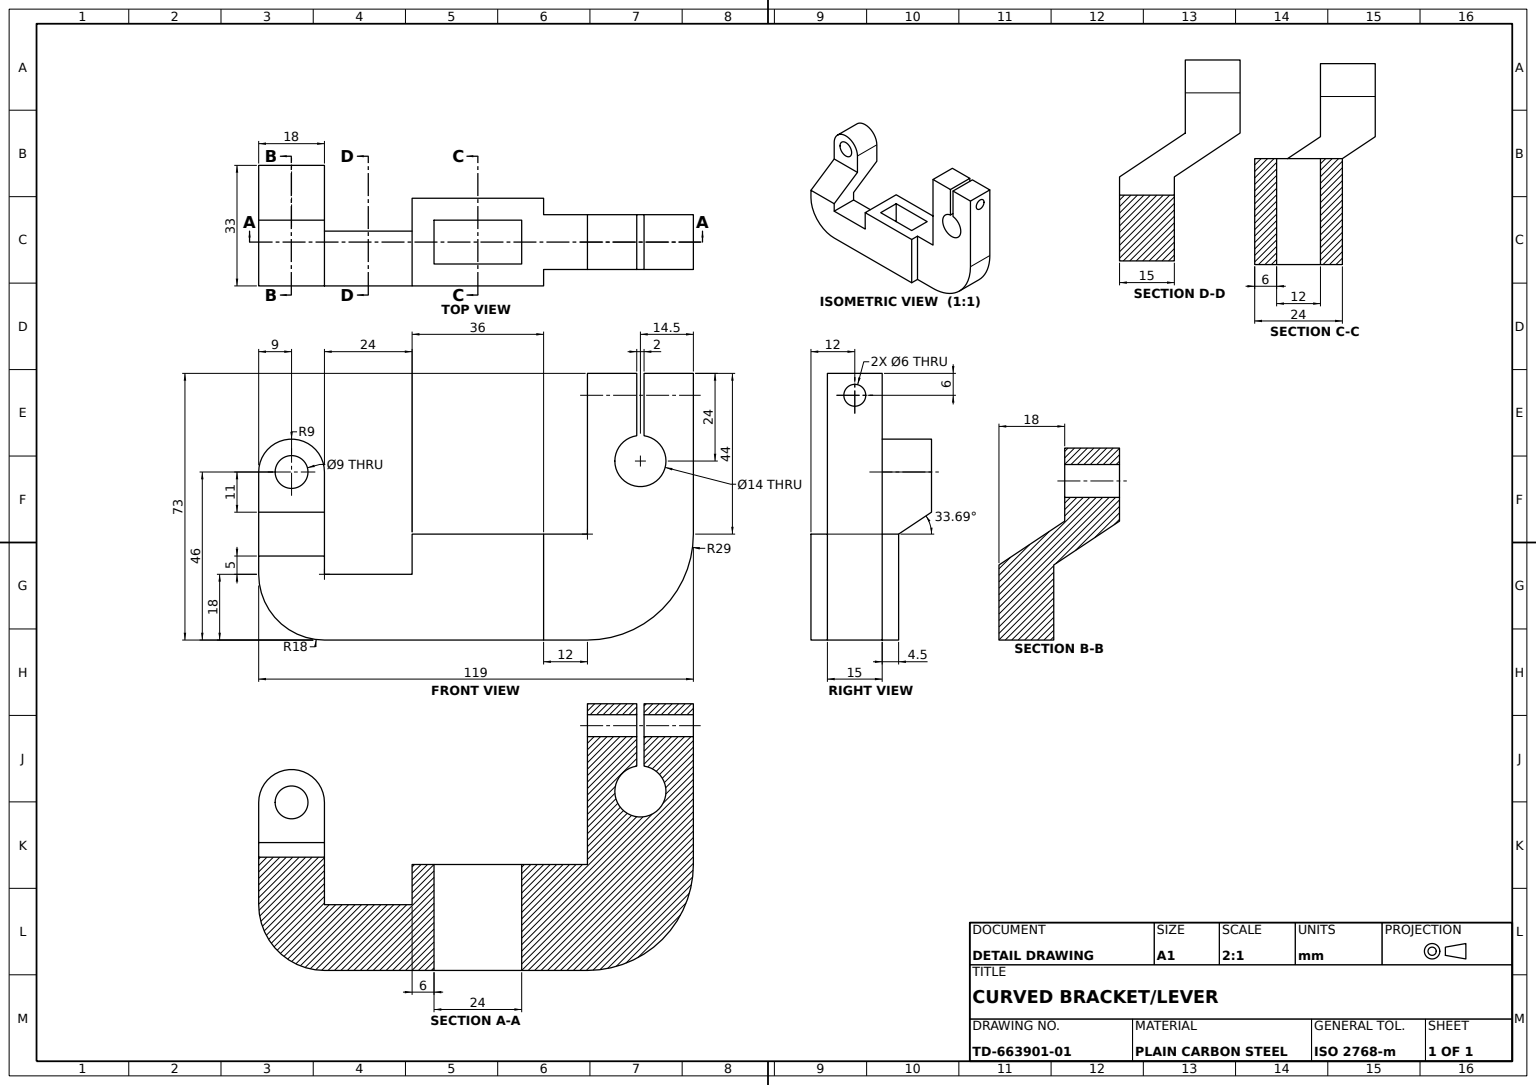
SolidWorks part; units mm, degrees
material "Plain Carbon Steel"
ref_plane "Front Plane" through (0, 0, 0) normal (0, 0, 1) x (1, 0, 0)
ref_plane "Top Plane" through (0, 0, 0) normal (0, 1, 0) x (1, 0, 0)
ref_plane "Right Plane" through (0, 0, 0) normal (1, 0, 0) x (0, 0, -1)
sketch "Bracket Profile Sketch" plane through (0, 0, 0) normal (0, 0, 1) x (1, 0, 0)
  line L0 (30, 14.5) -> (30, 58.5)
  line L1 (-18, -14.5) -> (18, -14.5)
  line L2 (-18, 3.5) -> (-18, 14.5)
  line L3 (-18, 14.5) -> (18, 14.5)
  line L5 (-18, -14.5) -> (18, 14.5) construction
  line L6 (-18, 14.5) -> (18, -14.5) construction
  line L7 (-18, -14.5) -> (-42, -14.5)
  line L9 (-18, 3.5) -> (-42, 3.5)
  line L10 (-42, -14.5) -> (-42, 3.5)
  line L11 (18, 14.5) -> (30, 14.5)
  line L13 (18, -14.5) -> (30, -14.5)
  line L15 (30, 58.5) -> (59, 58.5)
  line L16 (59, 58.5) -> (59, 14.5)
  arc A0 (59, 14.5) -> (30, -14.5) centre (30, 14.5) cw
  point P0 (0, 0)
  dimension "D8" = 29
  dimension "D1" = 36
  dimension "D2" = 29
  dimension "D3" = 24
  dimension "D4" = 18
  dimension "D5" = 18
  dimension "D6" = 12
  dimension "D7" = 44
  dimension "D9" = 29
  dimension "D10" = 14.5
extrude "Bracket Body" add sketch "Bracket Profile Sketch" along normal mid plane 24
sketch "Body Relief Sketch" plane through (0, 14.5, 0) normal (0, 1, 0) x (1, 0, 0)
  line L1 (-12, -6) -> (12, -6)
  line L2 (-12, -6) -> (-12, 6)
  line L3 (-12, 6) -> (12, 6)
  line L4 (12, -6) -> (12, 6)
  line L5 (-12, -6) -> (12, 6) construction
  line L6 (-12, 6) -> (12, -6) construction
  line L10 (-18, -12) -> (-18, 12) construction
  line L11 (-42, 12) -> (-18, 12)
  line L12 (-42, 12) -> (-42, 3)
  line L13 (-42, 3) -> (-18, 3)
  line L14 (-18, 12) -> (-18, 3)
  line L15 (-18, -12) -> (-42, -12) construction
  line L17 (59, -12) -> (18, -12)
  line L18 (59, -12) -> (59, -7.5)
  line L19 (59, -7.5) -> (18, -7.5)
  line L20 (18, -12) -> (18, -7.5)
  line L21 (59, -12) -> (59, 12) construction
  line L22 (18, 12) -> (59, 12)
  line L23 (18, 12) -> (18, 7.5)
  line L24 (18, 7.5) -> (59, 7.5)
  line L25 (59, 12) -> (59, 7.5)
  line L26 (30, -12) -> (30, 12) construction
  line L27 (30, 12) -> (-18, 12) construction
  point P0 (0, 0)
  dimension "D1" = 24
  dimension "D2" = 12
  dimension "D3" = 15
  dimension "D4" = 15
  dimension "D5" = 4.5
  dimension "D6" = 12
extrude "Body Relief Cut" cut sketch "Body Relief Sketch" against normal through all both and the other way through all
sketch "Window Sketch" plane through (0, 0, 7.5) normal (0, 0, 1) x (1, 0, 0)
  line L0 (59, 58.5) -> (30, 58.5) construction
  line L3 (43.5, 41.4282) -> (43.5, 58.5)
  line L4 (43.5, 58.5) -> (45.5, 58.5)
  line L5 (45.5, 41.4282) -> (45.5, 58.5)
  arc A0 (43.5, 41.4282) -> (45.5, 41.4282) centre (44.5, 34.5) ccw
  point P4 (44.5, 58.5)
  dimension "D1" = 14
  dimension "D2" = 24
  dimension "D3" = 2
extrude "Rectangular Window" cut sketch "Window Sketch" against normal through all
sketch "Clamp Hole Sketch" plane through (30, 0, 0) normal (-1, 0, 0) x (0, 0, 1)
  line L0 (7.5, 58.5) -> (-7.5, 58.5) construction
  circle A0 centre (0, 52.5) radius 3
  point P4 (0, 58.5)
  dimension "D1" = 6
  dimension "D2" = 6
extrude "Clamp Hole Ø6" cut sketch "Clamp Hole Sketch" against normal through all
sketch "Arm Sketch" plane through (0, 0, 12) normal (0, 0, 1) x (1, 0, 0)
  line L0 (-60, 3.5) -> (-60, 8.5)
  line L1 (-60, 8.5) -> (-42, 8.5)
  line L2 (-42, 8.5) -> (-42, 3.5)
  line L3 (-42, 3.5) -> (-42, -14.5)
  arc A0 (-42, -14.5) -> (-60, 3.5) centre (-42, 3.5) cw
  dimension "D1" = 5
extrude "Arm Boss" add sketch "Arm Sketch" against normal up to surface (15 mm away) up to face at (-30, -5.5, -3)
sketch "Pivot Lug Sketch" plane through (-60, 0, 0) normal (-1, 0, 0) x (0, 0, 1)
  line L0 (-3, 8.5) -> (-21, 20.5)
  line L2 (-6, 20.5) -> (12, 8.5)
  line L3 (12, 8.5) -> (-3, 8.5)
  line L4 (12, -14.5) -> (-3, -14.5) construction
  line L6 (-21, 20.5) -> (-21, 31.5)
  line L7 (-21, 31.5) -> (-6, 31.5)
  line L8 (-6, 20.5) -> (-6, 31.5)
  dimension "D1" = 18
  dimension "D2" = 15
  dimension "D3" = 11
  dimension "D4" = 46
extrude "Pivot Lug" add sketch "Pivot Lug Sketch" against normal up to surface (18 mm away) up to face at (-42, 6, 4.5)
sketch "Lug Fill Sketch" plane through (0, 0, -6) normal (0, 0, 1) x (1, 0, 0)
  line L0 (-42, 31.5) -> (-60, 31.5) construction
  line L1 (-60, 31.5) -> (-42, 31.5)
  arc A0 (-60, 31.5) -> (-42, 31.5) centre (-51, 31.5) cw
extrude "Lug Fill Boss" add sketch "Lug Fill Sketch" against normal up to surface (15 mm away) up to face at (-51, 26, -21)
sketch "Pivot Bore Sketch" plane through (0, 0, -6) normal (0, 0, 1) x (1, 0, 0)
  circle A0 centre (-51, 31.5) radius 4.5
  arc A1 (-42, 31.5) -> (-60, 31.5) centre (-51, 31.5) ccw construction
  dimension "D1" = 9
extrude "Pivot Bore Ø9" cut sketch "Pivot Bore Sketch" against normal blind 24
